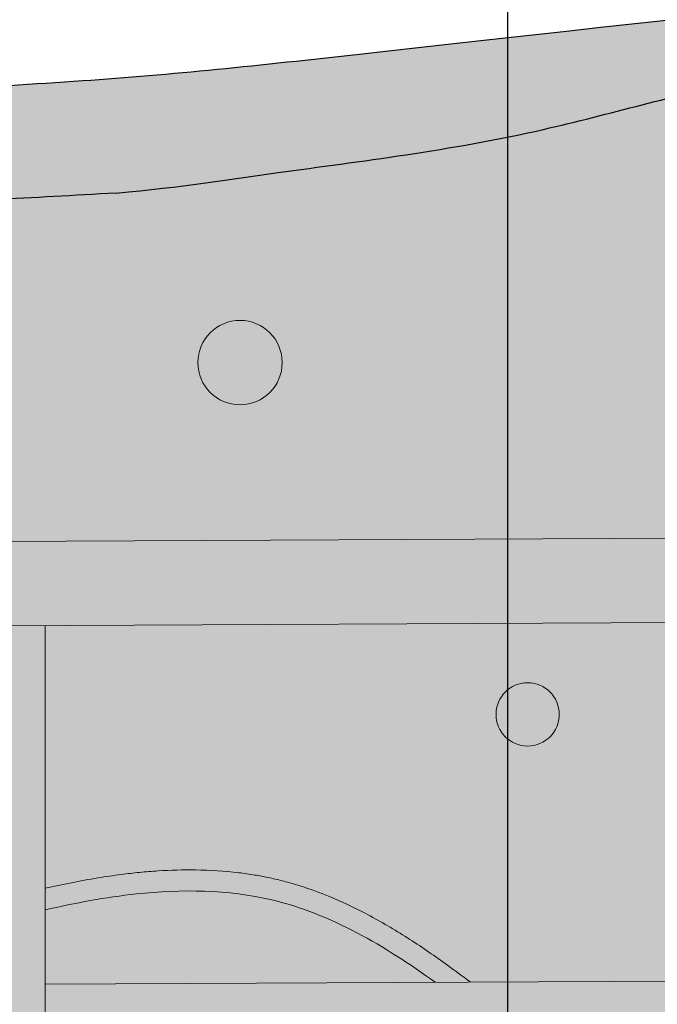
# Model space of a CAD drawing. Units: millimetres. Extents: x 11032 to 26788, y 3406 to 24505.
# Tile 66 of 78: x 19737 to 21249, y 15108 to 17443. Entities that reach past the tile are written whole.
import ezdxf

# ---------------------------------------------------------------- set-up
doc = ezdxf.new("R2010")
doc.units = ezdxf.units.MM
doc.header["$MEASUREMENT"] = 0
for name, color, linetype, lineweight in [('A-ANNO-DIMS', 2, 'Continuous', 18), ('A-GLAZ', 250, 'Continuous', 20), ('A-GLAZ-PATT', 9, 'Continuous', 13), ('A-ROOF', 7, 'Continuous', 30), ('E-LITE', 7, 'Continuous', 18), ('E-LITE-PATT', 7, 'Continuous', 13)]:
    doc.layers.add(name, color=color, linetype=linetype, lineweight=lineweight)
doc.layers.add('A-GLAZ-FRAM-PATT', color=250, linetype='Continuous', lineweight=13, true_color=0x262627)
doc.layers.add('A-ROOF-PATT', color=9, linetype='Continuous', lineweight=13, true_color=0xc7c8ca)
doc.styles.get("Standard").update_dxf_attribs({"font": 'arial.ttf'})
doc.dimstyles.get("Standard").update_dxf_attribs({"dimtxt": 150, "dimasz": 100, "dimexe": 10, "dimexo": 5, "dimgap": 5, "dimtad": 0, "dimtih": 1, "dimtoh": 1, "dimdec": 0, "dimzin": 0, "dimdsep": 46, "dimtxsty": 'Standard', "dimcen": 0.09, "dimadec": 0, "dimazin": 0, "dimtfac": 1, "dimtdec": 0, "dimtofl": 0, "dimtmove": 0, "dimatfit": 3, "dimfxl": 1, "dimtolj": 1, "dimtzin": 0, "dimarcsym": 0})

# ---------------------------------------------------------------- blocks, each defined once
blk = doc.blocks.new('RECESSED-LIGHT-150')
blk.add_circle((75, 75), 75)
blk = doc.blocks.new('RECESSED-LIGHT-200')
blk.add_circle((100, 100), 100)
blk = doc.blocks.new('*D36')
at = {"layer": 'A-ANNO-DIMS', "color": 0, "lineweight": -2, "transparency": 16777216}
for p, q in [((12301.3, 17115.9), (12301.3, 24416.9)), ((25397.4, 4466.4), (25397.4, 24416.9)), ((12401.3, 24406.9), (18569.2, 24406.9)), ((25297.4, 24406.9), (19129.5, 24406.9))]:
    blk.add_line(p, q, dxfattribs=at)
at = {"layer": 'A-ANNO-DIMS', "color": 0, "transparency": 16777216}
for points in [[(12401.3, 24423.5), (12401.3, 24390.2), (12301.3, 24406.9)], [(25297.4, 24423.5), (25297.4, 24390.2), (25397.4, 24406.9)]]:
    blk.add_solid(points, dxfattribs=at)
at = {"layer": 'Defpoints', "color": 0, "transparency": 16777216}
for p in [(25397.4, 24406.9), (12301.3, 17110.9), (25397.4, 4461.4)]:
    blk.add_point(p, dxfattribs=at)
at = {"layer": 'A-ANNO-DIMS', "color": 0, "transparency": 16777216, "insert": (18849.3, 24406.9), "char_height": 150, "attachment_point": 5}
blk.add_mtext('\\A1;13096', dxfattribs=at)
blk = doc.blocks.new('*D45')
at = {"layer": 'A-ANNO-DIMS', "color": 0, "lineweight": -2, "transparency": 16777216}
for p, q in [((13792.4, 18518.9), (26363.9, 18518.9)), ((26353.9, 18418.9), (26353.9, 17450.3)), ((26353.9, 16318.4), (26353.9, 17287)), ((22902.4, 16218.4), (26363.9, 16218.4))]:
    blk.add_line(p, q, dxfattribs=at)
at = {"layer": 'A-ANNO-DIMS', "color": 0, "transparency": 16777216}
for points in [[(26337.2, 18418.9), (26370.6, 18418.9), (26353.9, 18518.9)], [(26337.2, 16318.4), (26370.6, 16318.4), (26353.9, 16218.4)]]:
    blk.add_solid(points, dxfattribs=at)
at = {"layer": 'Defpoints', "color": 0, "transparency": 16777216}
for p in [(13787.4, 18518.9), (26353.9, 18518.9), (22897.4, 16218.4)]:
    blk.add_point(p, dxfattribs=at)
at = {"layer": 'A-ANNO-DIMS', "color": 0, "transparency": 16777216, "insert": (26353.9, 17368.7), "char_height": 150, "attachment_point": 5}
blk.add_mtext('\\A1;2300.5', dxfattribs=at)
blk = doc.blocks.new('*D51')
at = {"layer": 'A-ANNO-DIMS', "color": 0, "lineweight": -2, "transparency": 16777216}
for p, q in [((19697.4, 16000.7), (19697.4, 3494.9)), ((21997.4, 16011.6), (21997.4, 3494.9)), ((19797.4, 3504.9), (20617.4, 3504.9)), ((21897.4, 3504.9), (21077.4, 3504.9))]:
    blk.add_line(p, q, dxfattribs=at)
at = {"layer": 'A-ANNO-DIMS', "color": 0, "transparency": 16777216}
for points in [[(19797.4, 3521.6), (19797.4, 3488.2), (19697.4, 3504.9)], [(21897.4, 3521.6), (21897.4, 3488.2), (21997.4, 3504.9)]]:
    blk.add_solid(points, dxfattribs=at)
at = {"layer": 'Defpoints', "color": 0, "transparency": 16777216}
for p in [(21997.4, 16016.6), (19697.4, 16005.7), (21997.4, 3504.9)]:
    blk.add_point(p, dxfattribs=at)
at = {"layer": 'A-ANNO-DIMS', "color": 0, "transparency": 16777216, "insert": (20847.4, 3504.9), "char_height": 150, "attachment_point": 5}
blk.add_mtext('\\A1;2300', dxfattribs=at)
blk = doc.blocks.new('*D57')
at = {"layer": 'A-ANNO-DIMS', "color": 0, "lineweight": -2, "transparency": 16777216}
for p, q in [((14994.7, 7266.4), (14994.7, 24416.9)), ((20894.7, 7266.4), (20894.7, 24416.9)), ((15094.7, 24406.9), (17716, 24406.9)), ((20794.7, 24406.9), (18173.4, 24406.9))]:
    blk.add_line(p, q, dxfattribs=at)
at = {"layer": 'A-ANNO-DIMS', "color": 0, "transparency": 16777216}
for points in [[(15094.7, 24423.5), (15094.7, 24390.2), (14994.7, 24406.9)], [(20794.7, 24423.5), (20794.7, 24390.2), (20894.7, 24406.9)]]:
    blk.add_solid(points, dxfattribs=at)
at = {"layer": 'Defpoints', "color": 0, "transparency": 16777216}
for p in [(20894.7, 24406.9), (14994.7, 7261.4), (20894.7, 7261.4)]:
    blk.add_point(p, dxfattribs=at)
at = {"layer": 'A-ANNO-DIMS', "color": 0, "transparency": 16777216, "insert": (17944.7, 24406.9), "char_height": 150, "attachment_point": 5}
blk.add_mtext('\\A1;5900', dxfattribs=at)

msp = doc.modelspace()

# ---------------------------------------------------------------- hatches: boundary and pattern name
at = {"layer": 'A-GLAZ-FRAM-PATT'}
h = msp.add_hatch(color=256, dxfattribs=at)
h.paths.add_polyline_path([(22747.404, 16218.44), (22395.025, 16218.44), (18518.2, 16200.148), (18519.143, 16000.151), (22747.404, 16020.1)])
edge = h.paths.add_edge_path()
edge.add_line((22897.404, 16218.44), (22747.404, 16218.44))
edge.add_line((22747.404, 16218.44), (22747.404, 16020.1))
edge.add_line((22747.404, 16020.1), (22747.404, 9631.346))
edge.add_spline(control_points=[(22747.404, 9631.346), (22803.273, 9520.228), (22853.467, 9405.87), (22897.404, 9289.211)], knot_values=[2645.78092422, 2645.78092422, 2645.78092422, 2645.78092422, 3013.05623672, 3013.05623672, 3013.05623672, 3013.05623672], degree=3, periodic=0)
edge.add_line((22897.404, 9289.211), (22897.404, 16218.44))
h.paths.add_polyline_path([(22097.404, 16017.033), (21997.404, 16016.562), (21997.404, 13316.532), (22097.404, 13317.003)])
edge = h.paths.add_edge_path()
edge.add_line((19797.404, 16006.182), (19697.404, 16005.71))
edge.add_line((19697.404, 16005.71), (19697.404, 15155.703))
edge.add_line((19697.404, 15155.703), (19697.404, 12747.012))
edge.add_spline(control_points=[(19697.404, 12747.012), (19708.389, 12750.081), (19719.253, 12753.406), (19732.457, 12757.789), (19734.918, 12758.62), (19737.372, 12759.464)], knot_values=[1372.60477099, 1372.60477099, 1372.60477099, 1372.60477099, 1399.44343377, 1399.44343377, 1405.61279972, 1405.61279972, 1405.61279972, 1405.61279972], degree=3, periodic=0)
edge.add_spline(control_points=[(19737.372, 12759.464), (19750.245, 12763.891), (19762.932, 12768.657), (19778.9, 12775.14), (19782.354, 12776.572), (19785.794, 12778.028)], knot_values=[1405.61279972, 1405.61279972, 1405.61279972, 1405.61279972, 1437.96891336, 1437.96891336, 1446.94640473, 1446.94640473, 1446.94640473, 1446.94640473], degree=3, periodic=0)
edge.add_spline(control_points=[(19785.794, 12778.028), (19789.682, 12779.673), (19793.552, 12781.348), (19797.404, 12783.051)], knot_values=[1446.94640473, 1446.94640473, 1446.94640473, 1446.94640473, 1457.09545574, 1457.09545574, 1457.09545574, 1457.09545574], degree=3, periodic=0)
edge.add_line((19797.404, 12783.051), (19797.404, 15306.174))
edge.add_line((19797.404, 15306.174), (19797.404, 16006.182))
h = msp.add_hatch(color=256, dxfattribs=at)
h.paths.add_polyline_path([(19697.404, 15155.703), (18523.154, 15150.163), (18523.626, 15050.164), (19697.404, 15055.702)])
h.paths.add_polyline_path([(21997.404, 15166.555), (19797.404, 15156.175), (19797.404, 15056.174), (20912.335, 15061.434, -0.11801722), (20947.253, 15061.599), (21997.404, 15066.554)])
h.paths.add_polyline_path([(22747.404, 15170.094), (22097.404, 15167.027), (22097.404, 15067.026), (22747.404, 15070.092)])
edge = h.paths.add_edge_path()
edge.add_line((21997.404, 13241.531), (21332.397, 13238.393))
edge.add_spline(control_points=[(21332.397, 13238.393), (21338.038, 13214.902), (21343.139, 13191.382), (21354.5, 13132.481), (21360.029, 13097.149), (21368.306, 13027.119), (21371.052, 12992.421), (21373.63, 12924.101), (21373.462, 12890.481), (21370.61, 12834.187), (21368.665, 12811.15), (21365.955, 12788.546)], knot_values=[4470.65028407, 4470.65028407, 4470.65028407, 4470.65028407, 4531.4505555, 4531.4505555, 4623.16319106, 4623.16319106, 4714.87582662, 4714.87582662, 4806.58846218, 4806.58846218, 4871.89074498, 4871.89074498, 4871.89074498, 4871.89074498], degree=3, periodic=0)
edge.add_line((21365.955, 12788.546), (21997.404, 12791.526))
edge.add_line((21997.404, 12791.526), (21997.404, 13241.531))
h.paths.add_polyline_path([(22097.404, 13242.003), (21997.404, 13241.531), (21997.404, 12791.526), (22097.404, 12791.998)])
h.paths.add_polyline_path([(22697.404, 13244.833), (22097.404, 13242.003), (22097.404, 12791.998), (22697.404, 12794.828)])
at = {"layer": 'A-GLAZ-PATT'}
h = msp.add_hatch(color=256, dxfattribs=at)
h.set_gradient(color1=(254, 221, 154), color2=(248, 246, 176), name='CURVED')
edge = h.paths.add_edge_path()
edge.add_spline(control_points=[(18522.918, 15200.175), (18561.599, 15201.209), (18600.224, 15202.243), (18716.594, 15205.749), (18794.099, 15208.613), (18948.086, 15217.451), (19024.568, 15223.425), (19176.135, 15240.511), (19251.219, 15251.623), (19333.848, 15267.966), (19342.25, 15269.676), (19356.967, 15272.758), (19363.289, 15274.111), (19375.94, 15276.871), (19382.267, 15278.279), (19401.252, 15282.576), (19413.915, 15285.541), (19451.935, 15294.685), (19477.322, 15301.111), (19548.254, 15319.552), (19593.948, 15331.984), (19659.079, 15349.253), (19678.203, 15354.269), (19697.404, 15359.188)], knot_values=[1.09285599, 1.09285599, 1.09285599, 1.09285599, 116.34451384, 116.34451384, 349.03354152, 349.03354152, 581.72256921, 581.72256921, 814.41159689, 814.41159689, 840.78637359, 840.78637359, 860.67891922, 860.67891922, 880.57146485, 880.57146485, 920.35655611, 920.35655611, 999.92673863, 999.92673863, 1142.09604805, 1142.09604805, 1200.90860694, 1200.90860694, 1200.90860694, 1200.90860694], degree=3, periodic=0)
edge.add_line((19697.404, 15359.188), (19697.404, 16005.71))
edge.add_line((19697.404, 16005.71), (18519.143, 16000.151))
edge.add_line((18519.143, 16000.151), (18522.918, 15200.175))
edge = h.paths.add_edge_path()
edge.add_line((19697.404, 15055.702), (18523.626, 15050.164))
edge.add_line((18523.626, 15050.164), (18531.851, 13306.733))
edge.add_spline(control_points=[(18531.851, 13306.733), (18553.325, 13284.933), (18574.901, 13263.301), (18632.771, 13206.214), (18669.261, 13171.188), (18735.852, 13109.762), (18765.813, 13083.011), (18826.398, 13031.156), (18857.021, 13006.052), (18919.15, 12957.862), (18950.655, 12934.774), (19007.615, 12895.967), (19032.834, 12879.759), (19084.165, 12849.05), (19110.278, 12834.547), (19163.6, 12807.555), (19190.811, 12795.065), (19240.068, 12775.123), (19261.85, 12767.175), (19306.233, 12752.949), (19328.834, 12746.672), (19374.859, 12736.071), (19398.283, 12731.748), (19445.866, 12725.365), (19470.026, 12723.306), (19514.597, 12721.889), (19534.921, 12722.121), (19575.756, 12724.466), (19596.267, 12726.579), (19622.683, 12730.57), (19628.6, 12731.546), (19638.601, 12733.337), (19642.688, 12734.108), (19650.826, 12735.723), (19654.881, 12736.567), (19667.001, 12739.207), (19675.023, 12741.111), (19687.813, 12744.388), (19692.62, 12745.676), (19697.404, 12747.012)], knot_values=[259.28299856, 259.28299856, 259.28299856, 259.28299856, 332.45020059, 332.45020059, 454.53383699, 454.53383699, 552.84889009, 552.84889009, 651.16394319, 651.16394319, 749.47899629, 749.47899629, 825.6298474, 825.6298474, 901.7806985, 901.7806985, 977.9315496, 977.9315496, 1036.43952646, 1036.43952646, 1094.94750331, 1094.94750331, 1153.45548017, 1153.45548017, 1211.96345702, 1211.96345702, 1260.21270617, 1260.21270617, 1308.46195531, 1308.46195531, 1322.39247458, 1322.39247458, 1332.02384448, 1332.02384448, 1341.65521438, 1341.65521438, 1360.91795418, 1360.91795418, 1372.60477099, 1372.60477099, 1372.60477099, 1372.60477099], degree=3, periodic=0)
edge.add_line((19697.404, 12747.012), (19697.404, 15055.702))
h.paths.add_polyline_path([(18790.086, 14298.34, -1), (18890.086, 14298.34, -1)], flags=16)
h.paths.add_polyline_path([(19437.524, 14550.125, -1), (19537.524, 14550.125, -1)], flags=16)
h.paths.add_polyline_path([(22697.404, 16019.864), (22097.404, 16017.033), (22097.404, 15167.027), (22697.404, 15169.858)])
h.paths.add_polyline_path([(22697.404, 15069.857), (22097.404, 15067.026), (22097.404, 13317.003), (22697.404, 13319.834)])
h.paths.add_polyline_path([(20866.429, 15795.606, -1), (21016.429, 15795.606, -1)], flags=16)
h.paths.add_polyline_path([(19822.441, 15337.78), (19797.404, 15332.147), (19797.404, 15156.175), (20721.869, 15160.537), (20700.803, 15175.665), (20679.512, 15190.548), (20657.993, 15205.143), (20636.247, 15219.41), (20614.273, 15233.307), (20592.07, 15246.794), (20569.639, 15259.829), (20546.978, 15272.372), (20524.088, 15284.38), (20500.968, 15295.814), (20477.616, 15306.631), (20454.034, 15316.792), (20430.219, 15326.254), (20406.173, 15334.976), (20381.894, 15342.919), (20357.382, 15350.039), (20332.636, 15356.297), (20307.662, 15361.667), (20282.483, 15366.173), (20257.125, 15369.849), (20231.617, 15372.729), (20205.984, 15374.847), (20180.253, 15376.236), (20154.451, 15376.931), (20128.605, 15376.964), (20102.742, 15376.37), (20076.889, 15375.183), (20051.072, 15373.436), (20025.318, 15371.163), (19999.653, 15368.398), (19974.087, 15365.173), (19948.614, 15361.516), (19923.228, 15357.456), (19897.924, 15353.024), (19872.695, 15348.248), (19847.536, 15343.157)])
h.paths.add_polyline_path([(19797.404, 15383.428), (19822.666, 15388.998), (19848.044, 15394.311), (19873.542, 15399.338), (19899.168, 15404.048), (19924.927, 15408.41), (19950.824, 15412.396), (19976.865, 15415.972), (20003.054, 15419.109), (20029.394, 15421.774), (20055.871, 15423.934), (20082.461, 15425.553), (20109.142, 15426.594), (20135.888, 15427.02), (20162.676, 15426.794), (20189.481, 15425.88), (20216.28, 15424.237), (20243.046, 15421.828), (20269.754, 15418.614), (20296.377, 15414.554), (20322.887, 15409.61), (20349.254, 15403.74), (20375.368, 15396.947), (20401.163, 15389.283), (20426.64, 15380.795), (20451.799, 15371.531), (20476.643, 15361.538), (20501.172, 15350.863), (20525.391, 15339.55), (20549.302, 15327.645), (20572.91, 15315.192), (20596.218, 15302.234), (20619.229, 15288.816), (20641.948, 15274.978), (20664.378, 15260.764), (20686.523, 15246.215), (20708.386, 15231.373), (20729.97, 15216.279), (20751.277, 15200.974), (20806.33, 15160.935), (21997.404, 15166.555), (21997.404, 16016.562), (19797.404, 16006.182)])
at = {"layer": 'A-ROOF-PATT'}
h = msp.add_hatch(color=256, dxfattribs=at)
edge = h.paths.add_edge_path()
edge.add_spline(control_points=[(18514.126, 17063.566), (18809.773, 17038.521), (19288.07, 16988.339), (19761.843, 17020.464), (19965.955, 17031.58)], knot_values=[0, 0, 0, 0, 871.48115533, 1383.18424693, 1383.18424693, 1383.18424693, 1383.18424693], degree=3, periodic=0)
edge.add_spline(control_points=[(19965.955, 17031.58), (20122.484, 17046.068), (20408.011, 17091.181), (20910.567, 17150.246), (21440.234, 17310.172), (21915.866, 17351.508), (22364.272, 17406.622), (22705.353, 17409.356), (22912.577, 17410.967), (22981.194, 17409.426)], knot_values=[0, 0, 0, 0, 414.81784697, 1085.22788952, 1556.54039253, 2003.31216232, 2520.51919616, 2899.47011217, 3092.27759325, 3092.27759325, 3092.27759325, 3092.27759325], degree=3, periodic=0)
edge.add_spline(control_points=[(22981.194, 17409.426), (23026.355, 17412.719), (23070.675, 17406.134), (23179.968, 17412.17), (23244.326, 17403.734), (23304.873, 17403.391)], knot_values=[11756.28081343, 11756.28081343, 11756.28081343, 11756.28081343, 11879.15309498, 11879.15309498, 12065.87545546, 12065.87545546, 12065.87545546, 12065.87545546], degree=3, periodic=0)
edge.add_spline(control_points=[(23304.873, 17403.391), (23443.416, 17391.278), (23687.5, 17400.339), (23988.629, 17323.661), (24193.084, 17226.949), (24257.37, 17136.735), (24279.347, 17098.191)], knot_values=[0, 0, 0, 0, 412.75172359, 727.19040018, 931.86025321, 1064.01641738, 1064.01641738, 1064.01641738, 1064.01641738], degree=3, periodic=0)
edge.add_spline(control_points=[(24279.347, 17098.191), (24276.632, 17112.026), (24103.56, 17784.539), (21679.83, 17482.933), (20092.886, 17311.864), (19886.51, 17298.161)], knot_values=[9435.32329041, 9435.32329041, 9435.32329041, 9435.32329041, 9511.54858978, 13244.41643911, 13837.11981978, 13837.11981978, 13837.11981978, 13837.11981978], degree=3, periodic=0)
edge.add_spline(control_points=[(19886.51, 17298.161), (19770.33, 17290.447), (19654.15, 17282.732), (19537.97, 17275.018), (19460.41, 17269.868), (19382.851, 17264.718), (19305.291, 17259.568)], knot_values=[8878.9087223, 8878.9087223, 8878.9087223, 8878.9087223, 9212.57342317, 9212.57342317, 9212.57342317, 9435.32303857, 9435.32303857, 9435.32303857, 9435.32303857], degree=3, periodic=0)
edge.add_spline(control_points=[(19305.291, 17259.568), (19183.371, 17255.041), (18919.19, 17257.277), (18655.158, 17260.282), (18513.182, 17263.662)], knot_values=[568.98430855, 568.98430855, 568.98430855, 568.98430855, 934.97323186, 1361.07600794, 1361.07600794, 1361.07600794, 1361.07600794], degree=3, periodic=0)
edge.add_line((18513.182, 17263.662), (18514.126, 17063.566))
h = msp.add_hatch(color=256, dxfattribs=at)
h.set_gradient(color1=(254, 234, 185), color2=(254, 204, 102), name='HEMISPHERICAL')
edge = h.paths.add_edge_path()
edge.add_line((22395.025, 16218.44), (22897.404, 16218.44))
edge.add_line((22897.404, 16218.44), (22897.404, 14361.22))
edge.add_spline(control_points=[(22897.404, 14361.22), (23633.498, 15762.375), (24369.592, 16638.387), (24279.347, 17098.191)], knot_values=[13837.11981978, 13837.11981978, 13837.11981978, 13837.11981978, 16370.50452639, 16370.50452639, 16370.50452639, 16370.50452639], degree=3, periodic=0)
edge.add_spline(control_points=[(24279.347, 17098.191), (24257.37, 17136.735), (24193.084, 17226.949), (23988.629, 17323.661), (23687.5, 17400.339), (23443.416, 17391.278), (23304.873, 17403.391)], knot_values=[0, 0, 0, 0, 132.15616417, 336.8260172, 651.2646938, 1064.01641738, 1064.01641738, 1064.01641738, 1064.01641738], degree=3, periodic=0)
edge.add_spline(control_points=[(23304.873, 17403.391), (23244.326, 17403.734), (23179.968, 17412.17), (23070.675, 17406.134), (23026.355, 17412.719), (22981.194, 17409.426)], knot_values=[11756.28081343, 11756.28081343, 11756.28081343, 11756.28081343, 11943.0031739, 11943.0031739, 12065.87545546, 12065.87545546, 12065.87545546, 12065.87545546], degree=3, periodic=0)
edge.add_spline(control_points=[(22981.194, 17409.426), (22912.577, 17410.967), (22705.353, 17409.356), (22364.272, 17406.622), (21915.866, 17351.508), (21440.234, 17310.172), (20910.567, 17150.246), (20408.011, 17091.181), (20122.484, 17046.068), (19965.955, 17031.58)], knot_values=[0, 0, 0, 0, 192.80748108, 571.75839709, 1088.96543094, 1535.73720072, 2007.04970373, 2677.45974628, 3092.27759325, 3092.27759325, 3092.27759325, 3092.27759325], degree=3, periodic=0)
edge.add_spline(control_points=[(19965.955, 17031.58), (19761.843, 17020.464), (19288.07, 16988.339), (18809.773, 17038.521), (18514.126, 17063.566)], knot_values=[0, 0, 0, 0, 511.7030916, 1383.18424693, 1383.18424693, 1383.18424693, 1383.18424693], degree=3, periodic=0)
edge.add_line((18514.126, 17063.566), (18518.2, 16200.148))
edge.add_line((18518.2, 16200.148), (22395.025, 16218.44))
h.paths.add_polyline_path([(20159.481, 16629.671, -1), (20359.481, 16629.671, -1)], flags=16)
h.paths.add_polyline_path([(22641.869, 16640.848, -1), (22441.869, 16640.848, -1)], flags=16)
h.paths.add_polyline_path([(23436.23, 16026.079, -1), (23236.23, 16026.079, -1)], flags=16)
at = {"layer": 'E-LITE-PATT'}
h = msp.add_hatch(color=256, dxfattribs=at)
edge = h.paths.add_edge_path()
edge.add_spline(control_points=[(18523.154, 15150.163), (18807.347, 15157.761), (19206.112, 15168.423), (19587.098, 15279.026), (19697.404, 15307.557)], knot_values=[0, 0, 0, 0, 846.75149574, 1188.1141131, 1188.1141131, 1188.1141131, 1188.1141131], degree=3, periodic=0)
edge.add_line((19697.404, 15307.557), (19697.404, 15359.188))
edge.add_spline(control_points=[(19697.404, 15359.188), (19678.203, 15354.269), (19659.079, 15349.253), (19593.948, 15331.984), (19548.254, 15319.552), (19477.322, 15301.111), (19451.935, 15294.685), (19413.915, 15285.541), (19401.252, 15282.576), (19382.267, 15278.279), (19375.94, 15276.871), (19363.289, 15274.111), (19356.967, 15272.758), (19342.25, 15269.676), (19333.848, 15267.966), (19251.219, 15251.623), (19176.135, 15240.511), (19024.568, 15223.425), (18948.086, 15217.451), (18794.099, 15208.613), (18716.594, 15205.749), (18600.224, 15202.243), (18561.599, 15201.209), (18522.918, 15200.175)], knot_values=[1.09285599, 1.09285599, 1.09285599, 1.09285599, 59.90541488, 59.90541488, 202.0747243, 202.0747243, 281.64490682, 281.64490682, 321.42999808, 321.42999808, 341.32254371, 341.32254371, 361.21508934, 361.21508934, 387.58986604, 387.58986604, 620.27889372, 620.27889372, 852.96792141, 852.96792141, 1085.65694909, 1085.65694909, 1200.90860694, 1200.90860694, 1200.90860694, 1200.90860694], degree=3, periodic=0)
edge.add_line((18522.918, 15200.175), (18523.154, 15150.163))
edge = h.paths.add_edge_path()
edge.add_spline(control_points=[(19797.404, 15332.147), (19868.636, 15348.527), (20045.965, 15382.128), (20379.232, 15379.049), (20603.72, 15246.463), (20721.869, 15160.537)], knot_values=[1290.96802179, 1290.96802179, 1290.96802179, 1290.96802179, 1509.98304384, 1831.38750258, 2265.00925431, 2265.00925431, 2265.00925431, 2265.00925431], degree=3, periodic=0)
edge.add_line((20721.869, 15160.537), (20806.33, 15160.935))
edge.add_spline(control_points=[(20806.33, 15160.935), (20787.979, 15174.281), (20769.629, 15187.627), (20751.278, 15200.973), (20751.278, 15200.973), (20751.277, 15200.974), (20751.277, 15200.974)], knot_values=[2265.00925431, 2265.00925431, 2265.00925431, 2265.00925431, 2330.89307837, 2330.89307837, 2330.89307837, 2330.89358007, 2330.89358007, 2330.89358007, 2330.89358007], degree=3, periodic=0)
edge.add_spline(control_points=[(20751.277, 15200.974), (20751.247, 15200.996), (20751.217, 15201.018), (20722.252, 15222.081), (20692.553, 15242.645), (20631.556, 15281.877), (20600.258, 15300.544), (20535.977, 15335.007), (20502.992, 15350.803), (20448.844, 15372.942), (20428.246, 15380.535), (20396.869, 15390.701), (20386.329, 15393.886), (20370.401, 15398.335), (20365.072, 15399.763), (20354.373, 15402.506), (20349.001, 15403.822), (20337.544, 15406.494), (20331.459, 15407.834), (20315.169, 15411.216), (20304.944, 15413.125), (20281.909, 15416.972), (20269.086, 15418.802), (20222.263, 15424.425), (20188.116, 15426.504), (20124.362, 15427.321), (20094.738, 15426.456), (20050.592, 15423.632), (20035.925, 15422.435), (20006.724, 15419.587), (19992.193, 15417.937), (19959.175, 15413.705), (19940.732, 15410.994), (19880.215, 15401.109), (19838.589, 15392.722), (19797.404, 15383.428)], knot_values=[1302.24166378, 1302.24166378, 1302.24166378, 1302.24166378, 1302.35087893, 1302.35087893, 1406.225269, 1406.225269, 1510.09965908, 1510.09965908, 1613.97404916, 1613.97404916, 1676.17986117, 1676.17986117, 1707.28276717, 1707.28276717, 1722.83422018, 1722.83422018, 1738.38567318, 1738.38567318, 1755.91676333, 1755.91676333, 1785.22951081, 1785.22951081, 1821.79065604, 1821.79065604, 1918.47644845, 1918.47644845, 2002.64679624, 2002.64679624, 2044.73197014, 2044.73197014, 2086.81714404, 2086.81714404, 2140.81625119, 2140.81625119, 2265.00925431, 2265.00925431, 2265.00925431, 2265.00925431], degree=3, periodic=0)
edge.add_line((19797.404, 15383.428), (19797.404, 15332.147))
h.paths.add_polyline_path([(21016.429, 15795.606, 1), (20866.429, 15795.606, 1)])
h.paths.add_polyline_path([(23236.23, 16026.079, 1), (23436.23, 16026.079, 1)])
h.paths.add_polyline_path([(22441.869, 16640.848, 1), (22641.869, 16640.848, 1)])
h.paths.add_polyline_path([(20159.481, 16629.671, 1), (20359.481, 16629.671, 1)])

# ---------------------------------------------------------------- linework, layer by layer
at = {"layer": 'A-GLAZ'}
for p, q in [((22395.025, 16218.44), (18518.2, 16200.148)), ((22747.404, 16020.1), (18519.143, 16000.151)), ((19797.404, 16006.182), (19797.404, 15156.175)), ((19797.404, 15306.174), (19797.404, 12783.051)), ((21997.404, 15166.555), (19797.404, 15156.175))]:
    msp.add_line(p, q, dxfattribs=at)
at = {"layer": 'A-ROOF'}
for points, knots in [([(19305.291, 17259.568), (19382.851, 17264.718), (19460.41, 17269.868), (19537.97, 17275.018), (19654.15, 17282.732), (19770.33, 17290.447), (19886.51, 17298.161), (19886.51, 17298.161), (19886.51, 17298.161), (19886.51, 17298.161), (20092.886, 17311.864), (21679.83, 17482.933), (25498.5, 17958.124), (23655.645, 15804.534), (22897.404, 14361.22)], [8878.9087223, 8878.9087223, 8878.9087223, 8878.9087223, 9101.65833771, 9101.65833771, 9101.65833771, 9435.32303857, 9435.32303857, 9435.32303857, 9435.32329041, 9435.32329041, 9435.32329041, 10028.02667108, 13760.8945204, 16370.50452639, 16370.50452639, 16370.50452639, 16370.50452639]), ([(19965.955, 17031.58), (20122.484, 17046.068), (20408.011, 17091.181), (20910.567, 17150.246), (21440.234, 17310.172), (21915.866, 17351.508), (22364.272, 17406.622), (22705.353, 17409.356), (22912.577, 17410.967), (22981.194, 17409.426)], [0, 0, 0, 0, 414.81784697, 1085.22788952, 1556.54039253, 2003.31216232, 2520.51919616, 2899.47011217, 3092.27759325, 3092.27759325, 3092.27759325, 3092.27759325]), ([(19965.955, 17031.58), (19761.843, 17020.464), (19259.5, 16986.401), (18585.074, 17064.116), (18105.171, 17093.325), (17944.704, 17086.084)], [0, 0, 0, 0, 511.7030916, 1466.59375204, 1949.25960113, 1949.25960113, 1949.25960113, 1949.25960113])]:
    msp.add_open_spline(points, degree=3, knots=knots, dxfattribs=at)
at = {"layer": 'E-LITE'}
for points, knots in [([(19797.404, 15383.428), (19838.589, 15392.722), (19880.215, 15401.109), (19940.732, 15410.994), (19959.175, 15413.705), (19992.193, 15417.937), (20006.724, 15419.587), (20035.925, 15422.435), (20050.592, 15423.632), (20094.738, 15426.456), (20124.362, 15427.321), (20188.116, 15426.504), (20222.263, 15424.425), (20269.086, 15418.802), (20281.909, 15416.972), (20304.944, 15413.125), (20315.169, 15411.216), (20331.459, 15407.834), (20337.544, 15406.494), (20349.001, 15403.822), (20354.373, 15402.506), (20365.072, 15399.763), (20370.401, 15398.335), (20386.329, 15393.886), (20396.869, 15390.701), (20428.246, 15380.535), (20448.844, 15372.942), (20502.992, 15350.803), (20535.977, 15335.007), (20600.258, 15300.544), (20631.556, 15281.877), (20692.553, 15242.645), (20722.252, 15222.081), (20751.217, 15201.018), (20751.247, 15200.996), (20751.277, 15200.974), (20751.277, 15200.974), (20751.278, 15200.973), (20751.278, 15200.973), (20769.629, 15187.627), (20787.979, 15174.281), (20806.33, 15160.935)], [1302.24166378, 1302.24166378, 1302.24166378, 1302.24166378, 1426.4346669, 1426.4346669, 1480.43377405, 1480.43377405, 1522.51894795, 1522.51894795, 1564.60412184, 1564.60412184, 1648.77446964, 1648.77446964, 1745.46026205, 1745.46026205, 1782.02140728, 1782.02140728, 1811.33415476, 1811.33415476, 1828.86524491, 1828.86524491, 1844.41669791, 1844.41669791, 1859.96815091, 1859.96815091, 1891.07105692, 1891.07105692, 1953.27686893, 1953.27686893, 2057.15125901, 2057.15125901, 2161.02564908, 2161.02564908, 2264.90003916, 2264.90003916, 2265.00925431, 2265.00925431, 2265.00925431, 2265.00975601, 2265.00975601, 2265.00975601, 2330.89358007, 2330.89358007, 2330.89358007, 2330.89358007]), ([(19797.404, 15332.147), (19868.636, 15348.527), (20045.965, 15382.128), (20379.232, 15379.049), (20603.72, 15246.463), (20721.869, 15160.537)], [1290.96802179, 1290.96802179, 1290.96802179, 1290.96802179, 1509.98304384, 1831.38750258, 2265.00925431, 2265.00925431, 2265.00925431, 2265.00925431])]:
    msp.add_open_spline(points, degree=3, knots=knots, dxfattribs=at)

# ---------------------------------------------------------------- block references
for name, p in [('RECESSED-LIGHT-200', (20159.481, 16529.67)), ('RECESSED-LIGHT-150', (20866.429, 15720.606))]:
    msp.add_blockref(name, p, dxfattribs=at)

# ---------------------------------------------------------------- dimensions: what is measured, and where the dimension line sits
at = {"layer": 'A-ANNO-DIMS'}
for base, p1, p2, picture, middle in [((25397.404, 24406.858), (12301.265, 17110.885), (25397.404, 4461.399), '*D36', (18849.334, 24406.858)), ((20894.704, 24406.858), (14994.704, 7261.399), (20894.704, 7261.399), '*D57', (17944.704, 24406.858)), ((21997.404, 3504.899), (19697.404, 16005.71), (21997.404, 16016.562), '*D51', (20847.404, 3504.899))]:
    dim = msp.add_linear_dim(base=base, p1=p1, p2=p2, dimstyle='Standard', override={"dimdec": 0, "dimlfac": 1, "dimrnd": 0, "dimzin": 0, "dimdsep": 46, "dimlunit": 2}, dxfattribs=at)
    dim.commit()
    dim.dimension.update_dxf_attribs({"geometry": picture, "text_midpoint": middle})
dim = msp.add_linear_dim(base=(26353.904, 18518.925), p1=(22897.404, 16218.44), p2=(13787.367, 18518.925), angle=90, dimstyle='Standard', override={"dimdec": 1, "dimlfac": 1, "dimrnd": 0, "dimzin": 0, "dimdsep": 46, "dimlunit": 2}, dxfattribs=at)
dim.commit()
dim.dimension.update_dxf_attribs({"geometry": '*D45', "text_midpoint": (26353.904, 17368.682)})

doc.saveas('drawing.dxf')
